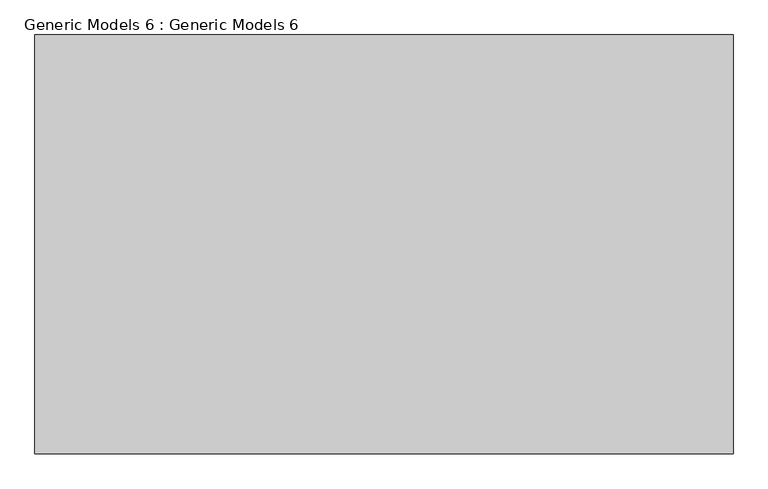
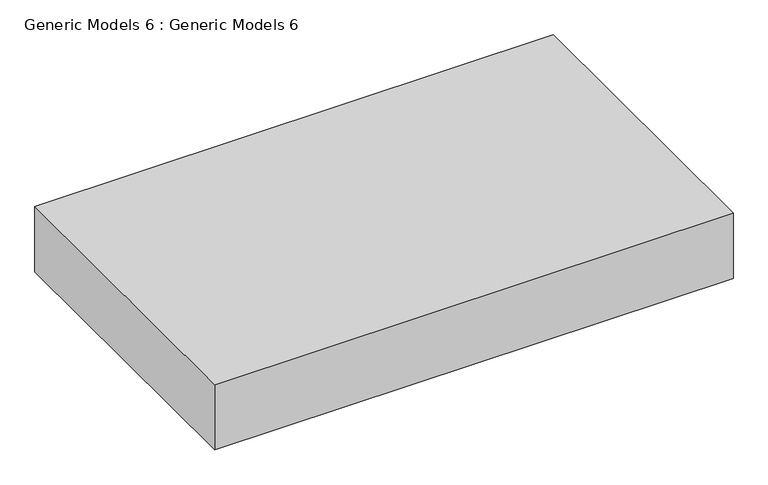
"""IFC4 building model written with IfcOpenShell, lengths in millimetres: proxy geometry, Generic Models 6 : Generic Models 6."""

from ifc_helpers import new_model, si_unit, frame, origin, place, context, project, spatial, polyline, outline, extrude, source, transform, mapped, element, save


def generic_models_6_generic_models_6_e57160bd(model_context):
    return source(origin(), model_context, "Body", "SweptSolid", [
        extrude(outline(polyline([(-8334.9678816, 2250.9030358), (-8334.9678816, 1336.5030358), (-9858.9678816, 1336.5030358), (-9858.9678816, 2250.9030358), (-8334.9678816, 2250.9030358)])), frame((0.0, 0.0, -203.2), z_axis=(0.0, 0.0, 1.0), x_axis=(1.0, 0.0, 0.0)), (0.0, 0.0, 1.0), 203.2),
    ])


if __name__ == "__main__":
    model = new_model("IFC4")
    model_context = context("Model", 3, world=origin())
    ifc_project = project(units=[si_unit("LENGTHUNIT", "METRE", prefix="MILLI")], contexts=[model_context])
    site = spatial("IfcSite", under=ifc_project)
    building = spatial("IfcBuilding", under=site)
    placement = place(None, origin())
    generic_models_6_generic_models_6_shape = generic_models_6_generic_models_6_e57160bd(model_context)
    element("IfcBuildingElementProxy", 1, Name="Generic Models 6 : Generic Models 6", ObjectType="Generic Models 6 : Generic Models 6", at=placement, inside=building, context=model_context, shape_type="MappedRepresentation", body=[
        mapped(generic_models_6_generic_models_6_shape, transform((0.0, 0.0, 0.0), x_axis=(1.0, 0.0, 0.0), y_axis=(0.0, 1.0, 0.0), z_axis=(0.0, 0.0, 1.0))),
    ])
    save(model, "model.ifc")

# Revit data of these elements
# Element 1 (IfcBuildingElementProxy, "Generic Models 6 : Generic Models 6")
#   Materials on its faces: "Concrete, Cast-in-Place gray"
# Materials
#   "Concrete, Cast-in-Place gray": class "Concrete", colour RGB 192 192 192, transparency 0, Description = "Cast-in-place concrete", Cost = 0
